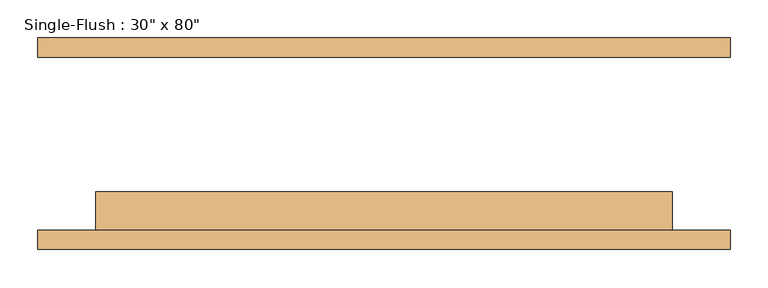
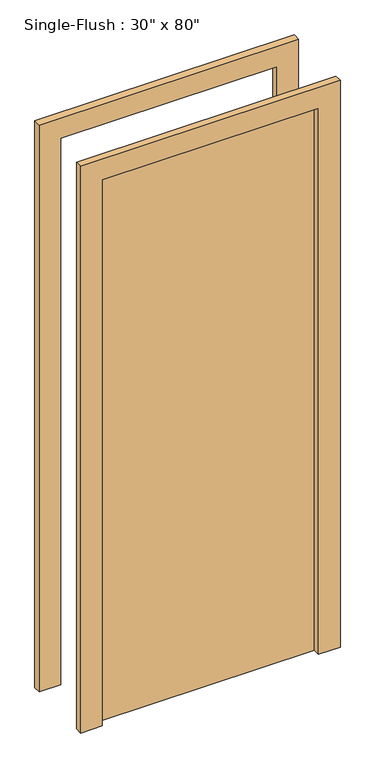
"""IFC4 building model written with IfcOpenShell, lengths in millimetres: door geometry."""

from ifc_helpers import new_model, si_unit, frame, origin, origin_with_axes, place, context, project, spatial, polyline, outline, extrude, source, transform, mapped, element, save


def door_85036156(model_context):
    return source(origin(), model_context, "Body", "SweptSolid", [
        extrude(outline(polyline([(2108.2, -457.2), (0.0, -457.2), (0.0, -381.0), (2032.0, -381.0), (2032.0, 381.0), (0.0, 381.0), (0.0, 457.2), (2108.2, 457.2), (2108.2, -457.2)])), frame((0.0, -139.7, 0.0), z_axis=(0.0, 1.0, 0.0), x_axis=(0.0, 0.0, 1.0)), (0.0, 0.0, 1.0), 25.4),
        extrude(outline(polyline([(2108.2, 457.2), (2108.2, -457.2), (0.0, -457.2), (0.0, -381.0), (2032.0, -381.0), (2032.0, 381.0), (0.0, 381.0), (0.0, 457.2), (2108.2, 457.2)])), frame((0.0, 114.3, 0.0), z_axis=(0.0, 1.0, 0.0), x_axis=(0.0, 0.0, 1.0)), (0.0, 0.0, 1.0), 25.4),
        extrude(outline(polyline([(381.0, -63.5), (381.0, -114.3), (-381.0, -114.3), (-381.0, -63.5), (381.0, -63.5)])), origin_with_axes(), (0.0, 0.0, 1.0), 2032.0),
    ])


if __name__ == "__main__":
    model = new_model("IFC4")
    model_context = context("Model", 3, world=origin())
    ifc_project = project(units=[si_unit("LENGTHUNIT", "METRE", prefix="MILLI")], contexts=[model_context])
    site = spatial("IfcSite", under=ifc_project)
    building = spatial("IfcBuilding", under=site)
    placement = place(None, origin())
    door_shape = door_85036156(model_context)
    element("IfcDoor", 1, ObjectType="Single-Flush : 30\" x 80\"", at=placement, inside=building, context=model_context, shape_type="MappedRepresentation", body=[
        mapped(door_shape, transform((0.0, 0.0, 0.0), x_axis=(1.0, 0.0, 0.0), y_axis=(0.0, 1.0, 0.0), z_axis=(0.0, 0.0, 1.0))),
    ])
    save(model, "model.ifc")

# Revit data of these elements
# Type "Single-Flush : 30\" x 80\""
#   Type Mark = "5"
#   Construction Type Id = "MDOOR"
#   Assembly Code = "C1020"
#   Analytic Construction = "Metal"
#   Thickness = 0' - 2"
#   Heat Transfer Coefficient (U) = 0.651978 BTU/(h·ft²·°F)
#   Height = 6' - 8"
#   Trim Projection Ext = 0' - 1"
#   Trim Projection Int = 0' - 1"
#   Trim Width = 0' - 3"
#   Width = 2' - 6"
#   Define Thermal Properties by = 1
#   Define Thermal Properties by = 1
#   Door Material = Door - Panel
#   Frame Material = Door - Frame
#   Visual Light Transmittance = 0
#   Solar Heat Gain Coefficient = 0
#   Function = (empty or 0)
#   Wall Closure = (empty or 0)
# Element 1 (IfcDoor, "Single-Flush : 30\" x 80\"")
#   Materials on its faces: "Door - Frame", "Door - Panel"
# Materials
#   "Door - Panel": class "Wood", colour RGB 210 159 95, transparency 0, Cost = 0
#   "Door - Frame": colour RGB 118 70 51, transparency 0, Cost = 0
